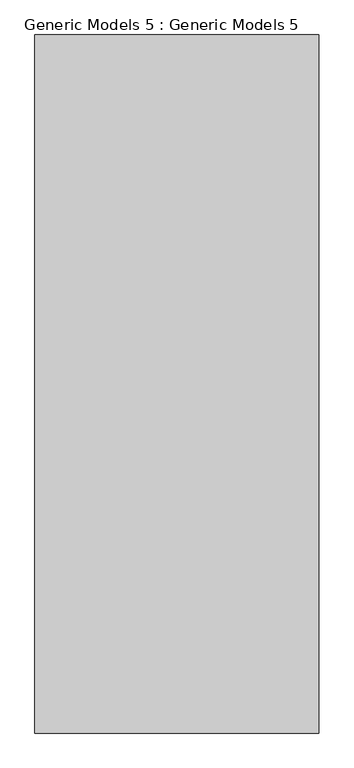
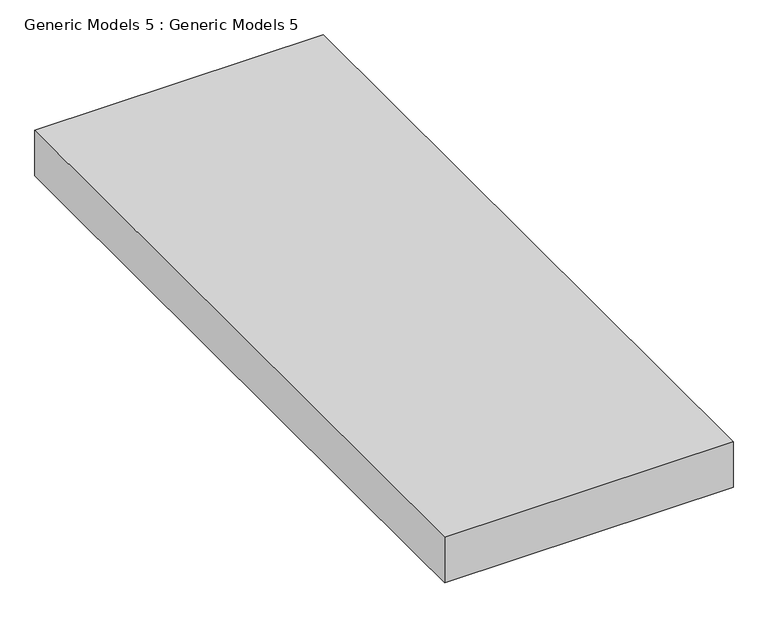
"""IFC4 building model written with IfcOpenShell, lengths in millimetres: proxy geometry, Generic Models 5 : Generic Models 5."""

from ifc_helpers import new_model, si_unit, frame, origin, place, context, project, spatial, polyline, outline, extrude, source, transform, mapped, element, save


def generic_models_5_generic_models_5_4455ebe8(model_context):
    return source(origin(), model_context, "Body", "SweptSolid", [
        extrude(outline(polyline([(12710.4756148, 2190.75), (12710.4756148, 2343.15), (14958.3756148, 2343.15), (14958.3756148, 2190.75), (14805.9756148, 2190.75), (12862.8756148, 2190.75), (12710.4756148, 2190.75)])), frame((-41311.6145004, 0.0, 0.0), z_axis=(1.0, 0.0, 0.0), x_axis=(0.0, 1.0, 0.0)), (0.0, 0.0, 1.0), 914.4),
    ])


if __name__ == "__main__":
    model = new_model("IFC4")
    model_context = context("Model", 3, world=origin())
    ifc_project = project(units=[si_unit("LENGTHUNIT", "METRE", prefix="MILLI")], contexts=[model_context])
    site = spatial("IfcSite", under=ifc_project)
    building = spatial("IfcBuilding", under=site)
    placement = place(None, origin())
    generic_models_5_generic_models_5_shape = generic_models_5_generic_models_5_4455ebe8(model_context)
    element("IfcBuildingElementProxy", 1, Name="Generic Models 5 : Generic Models 5", ObjectType="Generic Models 5 : Generic Models 5", at=placement, inside=building, context=model_context, shape_type="MappedRepresentation", body=[
        mapped(generic_models_5_generic_models_5_shape, transform((0.0, 0.0, 0.0), x_axis=(1.0, 0.0, 0.0), y_axis=(0.0, 1.0, 0.0), z_axis=(0.0, 0.0, 1.0))),
    ])
    save(model, "model.ifc")
